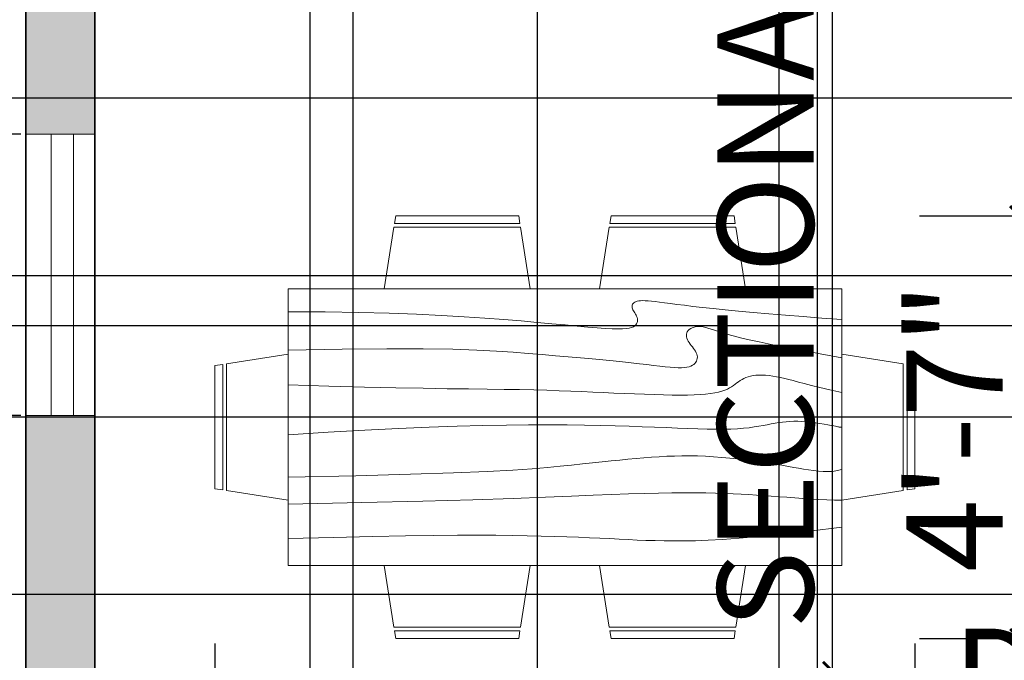
# Model space of a CAD drawing. Units: inches. Extents: x 1763 to 2368, y 1500 to 2097.
# Tile 6 of 24: x 1828 to 1956, y 1794 to 1877. Entities that reach past the tile are written whole.
import ezdxf

# ---------------------------------------------------------------- set-up
doc = ezdxf.new("R2010")
doc.units = ezdxf.units.IN
for name, color, linetype, lineweight in [('A-ANNO-DIMS', 2, 'Continuous', 18), ('A-FURN', 8, 'Continuous', 18), ('A-WALL', 7, 'Continuous', 35), ('A-WALL-PATT', 7, 'Continuous', 13), ('windows', 1, 'Continuous', 18)]:
    doc.layers.add(name, color=color, linetype=linetype, lineweight=lineweight)
doc.styles.get("Standard").update_dxf_attribs({"font": 'arial.ttf'})
doc.dimstyles.new('ISO-25', dxfattribs={"dimtxt": 12.5, "dimasz": 2.5, "dimexe": 1.25, "dimexo": 0.625, "dimtad": 1, "dimdec": 0, "dimlunit": 4, "dimtxsty": 'Standard', "dimblk": 'ARCHTICK', "dimcen": 2.5, "dimclrd": 3, "dimclrt": 4, "dimadec": 0, "dimazin": 0, "dimtfac": 1, "dimtdec": 0, "dimtmove": 0, "dimatfit": 3, "dimfxl": 1, "dimarcsym": 0})

# ---------------------------------------------------------------- blocks, each defined once
blk = doc.blocks.new('Dining Set - 36 x 72 in.')
for p, q in [((-22, 27.5), (-22.1562, 26.50042)), ((-22, 27.5), (-6, 27.5)), ((-5.8437, 26.49966), (-6, 27.5)), ((6, 27.5), (5.8438, 26.50042)), ((6, 27.5), (22, 27.5)), ((22.1563, 26.49966), (22, 27.5)), ((-22.2343, 26.00059), (-23.4847, 17.99762)), ((-22.2304, 26), (-5.7608, 26)), ((-5.8416, 26.5), (-22.1534, 26.5)), ((-4.5152, 17.99762), (-5.7655, 25.99926)), ((5.7657, 26.00059), (4.5153, 17.99762)), ((5.7696, 26), (22.2392, 26)), ((22.1584, 26.5), (5.8466, 26.5)), ((23.4848, 17.99762), (22.2345, 25.99926)), ((36, 18), (-36, 18)), ((-36, 18), (-36, -18)), ((36, -18), (36, 18)), ((-44.0006, 8.23428), (-35.9976, 9.48474)), ((44.0006, 8.23428), (35.9976, 9.48474)), ((-45.5, 8), (-44.5004, 8.15617)), ((-45.5, 8), (-45.5, -8)), ((-44.5, -8.15843), (-44.5, 8.15338)), ((-44, 8.23041), (-44, -8.23915)), ((44, 8.23041), (44, -8.23915)), ((44.5, -8.15843), (44.5, 8.15338)), ((45.5, 8), (44.5005, 8.15617)), ((45.5, 8), (45.5, -8)), ((-44.4997, -8.15631), (-45.5, -8)), ((-35.9976, -9.48476), (-43.9993, -8.2345)), ((35.9976, -9.48476), (43.9993, -8.2345)), ((44.4997, -8.15631), (45.5, -8)), ((-36, -18), (36, -18)), ((-22.2343, -26.0006), (-23.4847, -17.99762)), ((-4.5152, -17.99762), (-5.7655, -25.99928)), ((5.7657, -26.0006), (4.5153, -17.99762)), ((23.4848, -17.99762), (22.2345, -25.99928)), ((-22.2304, -26), (-5.7608, -26)), ((-22, -27.5), (-22.1562, -26.50044)), ((-5.8416, -26.5), (-22.1534, -26.5)), ((-5.8437, -26.49967), (-6, -27.5)), ((5.7696, -26), (22.2392, -26)), ((6, -27.5), (5.8438, -26.50044)), ((22.1584, -26.5), (5.8466, -26.5)), ((22.1563, -26.49967), (22, -27.5)), ((-22, -27.5), (-6, -27.5)), ((6, -27.5), (22, -27.5))]:
    blk.add_line(p, q)
for points in [[(-36, 15), (-31.1772, 14.97754), (-26.8079, 14.91406), (-22.8538, 14.81543), (-19.276, 14.6875), (-16.0362, 14.53613), (-13.0957, 14.36718), (-10.4159, 14.18652), (-7.9583, 14), (-5.6904, 13.81315), (-3.6035, 13.63021), (-1.6954, 13.45508), (0.0365, 13.29166), (1.5945, 13.14388), (2.9811, 13.01562), (4.1988, 12.9108), (5.25, 12.83333), (6.1393, 12.78613), (6.8802, 12.76823), (7.4883, 12.77767), (7.9792, 12.8125), (8.3685, 12.87077), (8.6719, 12.95052), (8.9049, 13.0498), (9.0833, 13.16666), (9.2205, 13.29899), (9.3216, 13.44401), (9.3895, 13.59879), (9.4271, 13.76041), (9.4373, 13.92594), (9.4232, 14.09245), (9.3875, 14.257), (9.3333, 14.41666), (9.2638, 14.56917), (9.1836, 14.71484), (9.0975, 14.85465), (9.0104, 14.98958), (8.9272, 15.1206), (8.8529, 15.2487), (8.7922, 15.37483), (8.75, 15.5), (8.7305, 15.62467), (8.7344, 15.74739), (8.7617, 15.86621), (8.8125, 15.97916), (8.8867, 16.08431), (8.9844, 16.17968), (9.1055, 16.26334), (9.25, 16.33333), (9.4189, 16.38802), (9.6172, 16.42708), (9.8506, 16.45052), (10.125, 16.45833), (10.4463, 16.45052), (10.8203, 16.42708), (11.2529, 16.38802), (11.75, 16.33333), (12.3184, 16.26318), (12.9694, 16.17838), (13.7151, 16.07991), (14.5677, 15.96875), (15.5395, 15.84586), (16.6426, 15.71224), (17.8893, 15.56884), (19.2917, 15.41666), (20.859, 15.25667), (22.5879, 15.08984), (24.4721, 14.91715), (26.5052, 14.73958), (28.6809, 14.5581), (30.9929, 14.3737), (33.4347, 14.18733), (36, 14)], [(-36, 10), (-28.9766, 10.14274), (-23.1725, 10.20442), (-18.4241, 10.19775), (-14.5677, 10.13541), (-11.4399, 10.03011), (-8.877, 9.89453), (-6.7154, 9.74137), (-4.7917, 9.58333), (-2.9698, 9.43082), (-1.2246, 9.28515), (0.4415, 9.14534), (2.026, 9.01041), (3.5266, 8.87939), (4.9408, 8.7513), (6.266, 8.62516), (7.5, 8.5), (8.6411, 8.37549), (9.6914, 8.2539), (10.6538, 8.13818), (11.5312, 8.03125), (12.3267, 7.93603), (13.043, 7.85547), (13.6831, 7.79248), (14.25, 7.75), (14.7471, 7.7303), (15.1797, 7.73307), (15.5537, 7.75732), (15.875, 7.80208), (16.1494, 7.86637), (16.3828, 7.94922), (16.5811, 8.04964), (16.75, 8.16666), (16.8944, 8.29915), (17.0143, 8.44531), (17.1089, 8.60319), (17.1771, 8.77083), (17.218, 8.94629), (17.2305, 9.1276), (17.2137, 9.31282), (17.1667, 9.5), (17.0895, 9.6875), (16.987, 9.875), (16.8649, 10.0625), (16.7292, 10.25), (16.5856, 10.4375), (16.4401, 10.625), (16.2985, 10.8125), (16.1667, 11), (16.05, 11.18733), (15.9518, 11.3737), (15.8752, 11.5581), (15.8229, 11.73958), (15.798, 11.91715), (15.8034, 12.08984), (15.842, 12.25667), (15.9167, 12.41666), (16.0295, 12.56836), (16.1784, 12.70833), (16.3605, 12.83268), (16.5729, 12.9375), (16.8127, 13.01888), (17.0768, 13.07291), (17.3625, 13.0957), (17.6667, 13.08333), (17.9894, 13.03312), (18.3418, 12.94726), (18.7382, 12.82918), (19.1927, 12.68229), (19.7195, 12.51001), (20.3327, 12.31575), (21.0465, 12.10294), (21.875, 11.875), (22.8357, 11.63354), (23.959, 11.37304), (25.2786, 11.08618), (26.8282, 10.76562), (28.6414, 10.40405), (30.752, 9.99414), (33.1936, 9.52856), (36, 9)], [(-36, 5.5), (-30.7157, 5.3348), (-26.069, 5.20963), (-21.9946, 5.11767), (-18.4271, 5.05208), (-15.3009, 5.00602), (-12.5508, 4.97265), (-10.1112, 4.94515), (-7.9167, 4.91666), (-5.909, 4.88167), (-4.0586, 4.83984), (-2.3429, 4.79215), (-0.7396, 4.73958), (0.7739, 4.6831), (2.22, 4.6237), (3.6213, 4.56233), (5, 4.5), (6.373, 4.43782), (7.7344, 4.3776), (9.0723, 4.32129), (10.375, 4.27083), (11.6309, 4.22819), (12.8281, 4.19531), (13.9551, 4.17415), (15, 4.16666), (15.954, 4.17448), (16.819, 4.19791), (17.6001, 4.23698), (18.3021, 4.29166), (18.9299, 4.36198), (19.4883, 4.44791), (19.9823, 4.54948), (20.4167, 4.66666), (20.7969, 4.79899), (21.1302, 4.94401), (21.4245, 5.09879), (21.6875, 5.26041), (21.9271, 5.42594), (22.1511, 5.59245), (22.3672, 5.757), (22.5834, 5.91666), (22.8065, 6.06868), (23.0404, 6.21093), (23.2879, 6.34147), (23.5521, 6.45833), (23.8358, 6.55957), (24.142, 6.64323), (24.4735, 6.70735), (24.8334, 6.75), (25.2235, 6.76969), (25.642, 6.76692), (26.0858, 6.74267), (26.5521, 6.69791), (27.0379, 6.63362), (27.5404, 6.55078), (28.0565, 6.45036), (28.5834, 6.33333), (29.1242, 6.19987), (29.7071, 6.04687), (30.3661, 5.87044), (31.1354, 5.66666), (32.0493, 5.43164), (33.142, 5.16146), (34.4475, 4.85221), (36, 4.5)], [(-36, -1), (-30.7915, -0.6591), (-26.0195, -0.38216), (-21.6519, -0.16284), (-17.6563, 0.00521), (-14.0005, 0.12833), (-10.6523, 0.21289), (-7.5796, 0.26522), (-4.75, 0.29166), (-2.134, 0.29793), (0.2878, 0.28711), (2.5317, 0.26163), (4.6146, 0.22396), (6.5529, 0.17651), (8.3633, 0.12174), (10.0623, 0.06209), (11.6667, 0), (13.1899, -0.06201), (14.6341, -0.1211), (15.9982, -0.17432), (17.2813, -0.21875), (18.4823, -0.25147), (19.6003, -0.26953), (20.6343, -0.27002), (21.5834, -0.25), (22.4481, -0.20768), (23.2357, -0.14584), (23.9549, -0.06836), (24.6146, 0.02083), (25.2235, 0.11784), (25.7904, 0.21875), (26.3241, 0.31966), (26.8334, 0.41666), (27.3265, 0.50618), (27.8099, 0.58593), (28.2894, 0.65397), (28.7709, 0.70833), (29.2601, 0.74707), (29.763, 0.76823), (30.2855, 0.76985), (30.8334, 0.75), (31.4088, 0.70784), (31.9994, 0.64713), (32.589, 0.57275), (33.1615, 0.48958), (33.7008, 0.4025), (34.1908, 0.3164), (34.6153, 0.23616), (34.9584, 0.16666), (35.2099, 0.11165), (35.3848, 0.07031), (35.504, 0.04069), (35.5886, 0.02083), (35.6594, 0.00879), (35.7377, 0.0026), (35.8442, 0.00032), (36, 0)], [(-36, -6.5), (-27.1843, -6.31267), (-20.084, -6.1263), (-14.469, -5.9419), (-10.1094, -5.76042), (-6.7752, -5.58285), (-4.2363, -5.41016), (-2.2629, -5.24333), (-0.625, -5.08334), (0.8708, -4.93099), (2.2715, -4.78646), (3.5872, -4.64974), (4.8281, -4.52084), (6.0046, -4.39974), (7.127, -4.28646), (8.2053, -4.18099), (9.25, -4.08334), (10.2705, -3.99382), (11.2734, -3.91407), (12.2647, -3.84603), (13.25, -3.79167), (14.2354, -3.75293), (15.2266, -3.73177), (16.2295, -3.73015), (17.25, -3.75), (18.2912, -3.79248), (19.3451, -3.85547), (20.4009, -3.93604), (21.4479, -4.03125), (22.4754, -4.13819), (23.4727, -4.25391), (24.4289, -4.37549), (25.3334, -4.5), (26.1785, -4.62492), (26.9694, -4.74935), (27.7145, -4.87281), (28.4219, -4.99479), (29.1, -5.11483), (29.7572, -5.23242), (30.4016, -5.34709), (31.0417, -5.45834), (31.6837, -5.56437), (32.3262, -5.65821), (32.9658, -5.73153), (33.599, -5.77604), (34.2224, -5.78345), (34.8327, -5.74545), (35.4264, -5.65373), (36, -5.5)], [(-36, -10), (-26.4022, -9.81299), (-18.4675, -9.62891), (-11.9839, -9.45069), (-6.7396, -9.28125), (-2.5226, -9.12354), (0.8789, -8.98047), (3.6769, -8.85498), (6.0833, -8.75), (8.2767, -8.66765), (10.3021, -8.60677), (12.1712, -8.56543), (13.8958, -8.54167), (15.4876, -8.53353), (16.9583, -8.53907), (18.3197, -8.55632), (19.5834, -8.58334), (20.7616, -8.61841), (21.8685, -8.66081), (22.9188, -8.71004), (23.9271, -8.76563), (24.9081, -8.82707), (25.8763, -8.89388), (26.8465, -8.96558), (27.8334, -9.04167), (28.8474, -9.12118), (29.8828, -9.20117), (30.93, -9.27824), (31.9792, -9.34896), (33.0205, -9.40991), (34.0443, -9.45768), (35.0407, -9.48885), (36, -9.5)], [(-36, -14.5), (-30.0881, -14.33513), (-25.0332, -14.21224), (-20.7312, -14.12647), (-17.0781, -14.07292), (-13.97, -14.04671), (-11.3027, -14.04297), (-8.9724, -14.05681), (-6.875, -14.08334), (-4.9224, -14.11833), (-3.0905, -14.16016), (-1.3709, -14.20785), (0.2448, -14.26042), (1.7647, -14.3169), (3.1973, -14.3763), (4.5507, -14.43767), (5.8333, -14.5), (7.0554, -14.5621), (8.235, -14.62175), (9.3922, -14.67652), (10.5469, -14.72396), (11.7192, -14.76164), (12.929, -14.78711), (14.1965, -14.79794), (15.5417, -14.79167), (16.9933, -14.76424), (18.6152, -14.70508), (20.4804, -14.60197), (22.6615, -14.44271), (25.2312, -14.21509), (28.2624, -13.9069), (31.8277, -13.50594), (36, -13)]]:
    blk.add_lwpolyline(points)
blk = doc.blocks.new('_ArchTick')
at = {"color": 0, "linetype": 'ByBlock', "const_width": 0.15}
blk.add_lwpolyline([(-0.5, -0.5), (0.5, 0.5)], dxfattribs=at)
blk = doc.blocks.new('*D25')
at = {"layer": 'A-ANNO-DIMS', "color": 3, "lineweight": -2, "transparency": 16777216}
for p, q in [((1934.01, 1792.31), (1934.01, 1981.61)), ((1934.01, 1660.94), (1934.01, 1792.31))]:
    blk.add_line(p, q, dxfattribs=at)
at = {"layer": 'A-ANNO-DIMS', "color": 0, "lineweight": -2, "transparency": 16777216}
for p, q in [((1953.09, 1792.31), (1932.76, 1792.31)), ((1953.09, 1660.94), (1932.76, 1660.94))]:
    blk.add_line(p, q, dxfattribs=at)
at = {"layer": 'Defpoints', "color": 0, "transparency": 16777216}
for p in [(1934.01, 1792.31), (1953.72, 1792.31), (1953.72, 1660.94)]:
    blk.add_point(p, dxfattribs=at)
at = {"layer": 'A-ANNO-DIMS', "color": 3, "lineweight": -2, "transparency": 16777216, "xscale": 2.5, "yscale": 2.5, "zscale": 2.5}
for p, rotation in [((1934.01, 1792.31), 90), ((1934.01, 1660.94), 270)]:
    blk.add_blockref('_ArchTick', p, dxfattribs=dict(at, rotation=rotation))
at = {"layer": 'A-ANNO-DIMS', "color": 4, "transparency": 16777216, "insert": (1926.92, 1888.21), "char_height": 12.5, "attachment_point": 5, "rotation": 90}
blk.add_mtext('SECTIONAL 10\'-11 1/2"', dxfattribs=at)
blk = doc.blocks.new('*D27')
at = {"layer": 'A-ANNO-DIMS', "color": 0, "lineweight": -2, "transparency": 16777216}
for p, q in [((1853.71, 1795.96), (1853.71, 1781.68)), ((1944.71, 1795.96), (1944.71, 1781.68))]:
    blk.add_line(p, q, dxfattribs=at)
at = {"layer": 'A-ANNO-DIMS', "color": 3, "lineweight": -2, "transparency": 16777216}
for p, q in [((1853.71, 1782.93), (1944.71, 1782.93)), ((1944.71, 1782.93), (2085.85, 1782.93))]:
    blk.add_line(p, q, dxfattribs=at)
at = {"layer": 'Defpoints', "color": 0, "transparency": 16777216}
for p in [(1853.71, 1796.58), (1944.71, 1796.58), (1944.71, 1782.93)]:
    blk.add_point(p, dxfattribs=at)
at = {"layer": 'A-ANNO-DIMS', "color": 3, "lineweight": -2, "transparency": 16777216, "xscale": 2.5, "yscale": 2.5, "zscale": 2.5, "rotation": 180}
blk.add_blockref('_ArchTick', (1853.71, 1782.93), dxfattribs=at)
at = {"layer": 'A-ANNO-DIMS', "color": 3, "lineweight": -2, "transparency": 16777216, "xscale": 2.5, "yscale": 2.5, "zscale": 2.5}
blk.add_blockref('_ArchTick', (1944.71, 1782.93), dxfattribs=at)
at = {"layer": 'A-ANNO-DIMS', "color": 4, "transparency": 16777216, "insert": (2016.53, 1790.02), "char_height": 12.5, "attachment_point": 5}
blk.add_mtext('DINING SET 7\'-7"', dxfattribs=at)
blk = doc.blocks.new('*D28')
at = {"layer": 'A-ANNO-DIMS', "color": 0, "lineweight": -2, "transparency": 16777216}
for p, q in [((1945.34, 1851.58), (1959.61, 1851.58)), ((1945.34, 1796.58), (1959.61, 1796.58))]:
    blk.add_line(p, q, dxfattribs=at)
at = {"layer": 'A-ANNO-DIMS', "color": 3, "lineweight": -2, "transparency": 16777216}
blk.add_line((1958.36, 1796.58), (1958.36, 1851.58), dxfattribs=at)
at = {"layer": 'Defpoints', "color": 0, "transparency": 16777216}
for p in [(1944.71, 1851.58), (1958.36, 1851.58), (1944.71, 1796.58)]:
    blk.add_point(p, dxfattribs=at)
at = {"layer": 'A-ANNO-DIMS', "color": 3, "lineweight": -2, "transparency": 16777216, "xscale": 2.5, "yscale": 2.5, "zscale": 2.5}
for p, rotation in [((1958.36, 1851.58), 90), ((1958.36, 1796.58), 270)]:
    blk.add_blockref('_ArchTick', p, dxfattribs=dict(at, rotation=rotation))
at = {"layer": 'A-ANNO-DIMS', "color": 4, "transparency": 16777216, "insert": (1951.49, 1824.08), "char_height": 12.5, "attachment_point": 5, "rotation": 90}
blk.add_mtext('4\'-7"', dxfattribs=at)
blk = doc.blocks.new('*D47')
at = {"layer": 'A-ANNO-DIMS', "color": 0, "lineweight": -2, "transparency": 16777216}
for p, q in [((1828.47, 1825.59), (1787.6, 1825.59)), ((1828.47, 1738.64), (1787.6, 1738.64))]:
    blk.add_line(p, q, dxfattribs=at)
at = {"layer": 'A-ANNO-DIMS', "color": 3, "lineweight": -2, "transparency": 16777216}
blk.add_line((1788.85, 1738.64), (1788.85, 1825.59), dxfattribs=at)
at = {"layer": 'Defpoints', "color": 0, "transparency": 16777216}
for p in [(1788.85, 1825.59), (1829.09, 1825.59), (1829.09, 1738.64)]:
    blk.add_point(p, dxfattribs=at)
at = {"layer": 'A-ANNO-DIMS', "color": 3, "lineweight": -2, "transparency": 16777216, "xscale": 2.5, "yscale": 2.5, "zscale": 2.5}
for p, rotation in [((1788.85, 1825.59), 90), ((1788.85, 1738.64), 270)]:
    blk.add_blockref('_ArchTick', p, dxfattribs=dict(at, rotation=rotation))
at = {"layer": 'A-ANNO-DIMS', "color": 4, "transparency": 16777216, "insert": (1781.84, 1782.12), "char_height": 12.5, "attachment_point": 5, "rotation": 90}
blk.add_mtext('7\'-3"', dxfattribs=at)
blk = doc.blocks.new('*D48')
at = {"layer": 'A-ANNO-DIMS', "color": 3, "lineweight": -2, "transparency": 16777216}
for p, q in [((1788.85, 1862.2), (1788.85, 1928.3)), ((1788.85, 1825.59), (1788.85, 1862.2))]:
    blk.add_line(p, q, dxfattribs=at)
at = {"layer": 'A-ANNO-DIMS', "color": 0, "lineweight": -2, "transparency": 16777216}
for p, q in [((1828.47, 1862.2), (1787.6, 1862.2)), ((1828.47, 1825.59), (1787.6, 1825.59))]:
    blk.add_line(p, q, dxfattribs=at)
at = {"layer": 'Defpoints', "color": 0, "transparency": 16777216}
for p in [(1788.85, 1862.2), (1829.09, 1862.2), (1829.09, 1825.59)]:
    blk.add_point(p, dxfattribs=at)
at = {"layer": 'A-ANNO-DIMS', "color": 3, "lineweight": -2, "transparency": 16777216, "xscale": 2.5, "yscale": 2.5, "zscale": 2.5}
for p, rotation in [((1788.85, 1862.2), 90), ((1788.85, 1825.59), 270)]:
    blk.add_blockref('_ArchTick', p, dxfattribs=dict(at, rotation=rotation))
at = {"layer": 'A-ANNO-DIMS', "color": 4, "transparency": 16777216, "insert": (1781.76, 1896.5), "char_height": 12.5, "attachment_point": 5, "rotation": 90}
blk.add_mtext('3\'-0 1/2"', dxfattribs=at)
blk = doc.blocks.new('*D49')
at = {"layer": 'A-ANNO-DIMS', "color": 0, "lineweight": -2, "transparency": 16777216}
for p, q in [((1828.47, 1913.1), (1787.6, 1913.1)), ((1828.47, 1862.2), (1787.6, 1862.2))]:
    blk.add_line(p, q, dxfattribs=at)
at = {"layer": 'A-ANNO-DIMS', "color": 3, "lineweight": -2, "transparency": 16777216}
blk.add_line((1788.85, 1862.2), (1788.85, 1913.1), dxfattribs=at)
at = {"layer": 'Defpoints', "color": 0, "transparency": 16777216}
for p in [(1788.85, 1913.1), (1829.09, 1913.1), (1829.09, 1862.2)]:
    blk.add_point(p, dxfattribs=at)
at = {"layer": 'A-ANNO-DIMS', "color": 3, "lineweight": -2, "transparency": 16777216, "xscale": 2.5, "yscale": 2.5, "zscale": 2.5}
for p, rotation in [((1788.85, 1913.1), 90), ((1788.85, 1862.2), 270)]:
    blk.add_blockref('_ArchTick', p, dxfattribs=dict(at, rotation=rotation))
at = {"layer": 'A-ANNO-DIMS', "color": 4, "transparency": 16777216, "insert": (1781.84, 1887.65), "char_height": 12.5, "attachment_point": 5, "rotation": 90}
blk.add_mtext('4\'-3"', dxfattribs=at)
blk = doc.blocks.new('*D58')
at = {"layer": 'A-ANNO-DIMS', "color": 0, "lineweight": -2, "transparency": 16777216}
for p, q in [((1871.68, 1635.9), (1871.68, 2072.02)), ((1927.07, 1635.9), (1927.07, 2072.02))]:
    blk.add_line(p, q, dxfattribs=at)
at = {"layer": 'A-ANNO-DIMS', "color": 3, "lineweight": -2, "transparency": 16777216}
for p, q in [((1871.68, 2070.77), (1927.07, 2070.77)), ((1927.07, 2070.77), (1993.68, 2070.77))]:
    blk.add_line(p, q, dxfattribs=at)
at = {"layer": 'Defpoints', "color": 0, "transparency": 16777216}
for p in [(1927.07, 2070.77), (1871.68, 1635.27), (1927.07, 1635.27)]:
    blk.add_point(p, dxfattribs=at)
at = {"layer": 'A-ANNO-DIMS', "color": 3, "lineweight": -2, "transparency": 16777216, "xscale": 2.5, "yscale": 2.5, "zscale": 2.5, "rotation": 180}
blk.add_blockref('_ArchTick', (1871.68, 2070.77), dxfattribs=at)
at = {"layer": 'A-ANNO-DIMS', "color": 3, "lineweight": -2, "transparency": 16777216, "xscale": 2.5, "yscale": 2.5, "zscale": 2.5}
blk.add_blockref('_ArchTick', (1927.07, 2070.77), dxfattribs=at)
at = {"layer": 'A-ANNO-DIMS', "color": 4, "transparency": 16777216, "insert": (1961.63, 2077.86), "char_height": 12.5, "attachment_point": 5}
blk.add_mtext('4\'-7 1/2"', dxfattribs=at)
blk = doc.blocks.new('*D68')
at = {"layer": 'A-ANNO-DIMS', "color": 0, "lineweight": -2, "transparency": 16777216}
for p, q in [((1895.59, 1879.65), (1895.59, 1509.91)), ((1932.01, 1879.65), (1932.01, 1509.91))]:
    blk.add_line(p, q, dxfattribs=at)
at = {"layer": 'A-ANNO-DIMS', "color": 3, "lineweight": -2, "transparency": 16777216}
for p, q in [((1895.59, 1511.16), (1932.01, 1511.16)), ((1932.01, 1511.16), (1998.11, 1511.16))]:
    blk.add_line(p, q, dxfattribs=at)
at = {"layer": 'Defpoints', "color": 0, "transparency": 16777216}
for p in [(1895.59, 1880.27), (1932.01, 1880.27), (1932.01, 1511.16)]:
    blk.add_point(p, dxfattribs=at)
at = {"layer": 'A-ANNO-DIMS', "color": 3, "lineweight": -2, "transparency": 16777216, "xscale": 2.5, "yscale": 2.5, "zscale": 2.5, "rotation": 180}
blk.add_blockref('_ArchTick', (1895.59, 1511.16), dxfattribs=at)
at = {"layer": 'A-ANNO-DIMS', "color": 3, "lineweight": -2, "transparency": 16777216, "xscale": 2.5, "yscale": 2.5, "zscale": 2.5}
blk.add_blockref('_ArchTick', (1932.01, 1511.16), dxfattribs=at)
at = {"layer": 'A-ANNO-DIMS', "color": 4, "transparency": 16777216, "insert": (1966.31, 1518.25), "char_height": 12.5, "attachment_point": 5}
blk.add_mtext('3\'-0 1/2"', dxfattribs=at)
blk = doc.blocks.new('*D69')
at = {"layer": 'A-ANNO-DIMS', "color": 0, "lineweight": -2, "transparency": 16777216}
for p, q in [((1838.09, 1879.65), (1838.09, 1509.91)), ((1895.59, 1879.65), (1895.59, 1509.91))]:
    blk.add_line(p, q, dxfattribs=at)
at = {"layer": 'A-ANNO-DIMS', "color": 3, "lineweight": -2, "transparency": 16777216}
for p, q in [((1838.09, 1511.16), (1895.59, 1511.16)), ((1895.59, 1511.16), (1962.2, 1511.16))]:
    blk.add_line(p, q, dxfattribs=at)
at = {"layer": 'Defpoints', "color": 0, "transparency": 16777216}
for p in [(1838.09, 1880.27), (1895.59, 1880.27), (1895.59, 1511.16)]:
    blk.add_point(p, dxfattribs=at)
at = {"layer": 'A-ANNO-DIMS', "color": 3, "lineweight": -2, "transparency": 16777216, "xscale": 2.5, "yscale": 2.5, "zscale": 2.5, "rotation": 180}
blk.add_blockref('_ArchTick', (1838.09, 1511.16), dxfattribs=at)
at = {"layer": 'A-ANNO-DIMS', "color": 3, "lineweight": -2, "transparency": 16777216, "xscale": 2.5, "yscale": 2.5, "zscale": 2.5}
blk.add_blockref('_ArchTick', (1895.59, 1511.16), dxfattribs=at)
at = {"layer": 'A-ANNO-DIMS', "color": 4, "transparency": 16777216, "insert": (1930.15, 1518.24), "char_height": 12.5, "attachment_point": 5}
blk.add_mtext('4\'-9 1/2"', dxfattribs=at)
blk = doc.blocks.new('*D79')
at = {"layer": 'A-ANNO-DIMS', "color": 3, "lineweight": -2, "transparency": 16777216}
for p, q in [((1788.85, 1825.4), (1788.85, 1870.91)), ((1788.85, 1802.3), (1788.85, 1825.4))]:
    blk.add_line(p, q, dxfattribs=at)
at = {"layer": 'A-ANNO-DIMS', "color": 0, "lineweight": -2, "transparency": 16777216}
for p, q in [((2054.47, 1825.4), (1787.6, 1825.4)), ((2054.47, 1802.3), (1787.6, 1802.3))]:
    blk.add_line(p, q, dxfattribs=at)
at = {"layer": 'Defpoints', "color": 0, "transparency": 16777216}
for p in [(1788.85, 1825.4), (2055.09, 1825.4), (2055.09, 1802.3)]:
    blk.add_point(p, dxfattribs=at)
at = {"layer": 'A-ANNO-DIMS', "color": 3, "lineweight": -2, "transparency": 16777216, "xscale": 2.5, "yscale": 2.5, "zscale": 2.5}
for p, rotation in [((1788.85, 1825.4), 90), ((1788.85, 1802.3), 270)]:
    blk.add_blockref('_ArchTick', p, dxfattribs=dict(at, rotation=rotation))
at = {"layer": 'A-ANNO-DIMS', "color": 4, "transparency": 16777216, "insert": (1781.95, 1849.4), "char_height": 12.5, "attachment_point": 5, "rotation": 90}
blk.add_mtext('1\'-11"', dxfattribs=at)
blk = doc.blocks.new('*D80')
at = {"layer": 'A-ANNO-DIMS', "color": 3, "lineweight": -2, "transparency": 16777216}
for p, q in [((1788.85, 1837.27), (1788.85, 1873.07)), ((1788.85, 1825.4), (1788.85, 1837.27))]:
    blk.add_line(p, q, dxfattribs=at)
at = {"layer": 'A-ANNO-DIMS', "color": 0, "lineweight": -2, "transparency": 16777216}
for p, q in [((2054.47, 1837.27), (1787.6, 1837.27)), ((2054.47, 1825.4), (1787.6, 1825.4))]:
    blk.add_line(p, q, dxfattribs=at)
at = {"layer": 'Defpoints', "color": 0, "transparency": 16777216}
for p in [(1788.85, 1837.27), (2055.09, 1837.27), (2055.09, 1825.4)]:
    blk.add_point(p, dxfattribs=at)
at = {"layer": 'A-ANNO-DIMS', "color": 3, "lineweight": -2, "transparency": 16777216, "xscale": 2.5, "yscale": 2.5, "zscale": 2.5}
for p, rotation in [((1788.85, 1837.27), 90), ((1788.85, 1825.4), 270)]:
    blk.add_blockref('_ArchTick', p, dxfattribs=dict(at, rotation=rotation))
at = {"layer": 'A-ANNO-DIMS', "color": 4, "transparency": 16777216, "insert": (1781.85, 1856.42), "char_height": 12.5, "attachment_point": 5, "rotation": 90}
blk.add_mtext('1\'-0"', dxfattribs=at)
blk = doc.blocks.new('*D81')
at = {"layer": 'A-ANNO-DIMS', "color": 3, "lineweight": -2, "transparency": 16777216}
for p, q in [((1788.85, 1866.87), (1788.85, 1912.38)), ((1788.85, 1843.77), (1788.85, 1866.87))]:
    blk.add_line(p, q, dxfattribs=at)
at = {"layer": 'A-ANNO-DIMS', "color": 0, "lineweight": -2, "transparency": 16777216}
for p, q in [((2077.47, 1866.87), (1787.6, 1866.87)), ((2077.47, 1843.77), (1787.6, 1843.77))]:
    blk.add_line(p, q, dxfattribs=at)
at = {"layer": 'Defpoints', "color": 0, "transparency": 16777216}
for p in [(1788.85, 1866.87), (2078.09, 1866.87), (2078.09, 1843.77)]:
    blk.add_point(p, dxfattribs=at)
at = {"layer": 'A-ANNO-DIMS', "color": 3, "lineweight": -2, "transparency": 16777216, "xscale": 2.5, "yscale": 2.5, "zscale": 2.5}
for p, rotation in [((1788.85, 1866.87), 90), ((1788.85, 1843.77), 270)]:
    blk.add_blockref('_ArchTick', p, dxfattribs=dict(at, rotation=rotation))
at = {"layer": 'A-ANNO-DIMS', "color": 4, "transparency": 16777216, "insert": (1781.95, 1890.87), "char_height": 12.5, "attachment_point": 5, "rotation": 90}
blk.add_mtext('1\'-11"', dxfattribs=at)
blk = doc.blocks.new('*D82')
at = {"layer": 'A-ANNO-DIMS', "color": 3, "lineweight": -2, "transparency": 16777216}
for p, q in [((1788.85, 1843.77), (1788.85, 1909.87)), ((1788.85, 1837.27), (1788.85, 1843.77))]:
    blk.add_line(p, q, dxfattribs=at)
at = {"layer": 'A-ANNO-DIMS', "color": 0, "lineweight": -2, "transparency": 16777216}
for p, q in [((2077.47, 1843.77), (1787.6, 1843.77)), ((2077.47, 1837.27), (1787.6, 1837.27))]:
    blk.add_line(p, q, dxfattribs=at)
at = {"layer": 'Defpoints', "color": 0, "transparency": 16777216}
for p in [(1788.85, 1843.77), (2078.09, 1843.77), (2078.09, 1837.27)]:
    blk.add_point(p, dxfattribs=at)
at = {"layer": 'A-ANNO-DIMS', "color": 3, "lineweight": -2, "transparency": 16777216, "xscale": 2.5, "yscale": 2.5, "zscale": 2.5}
for p, rotation in [((1788.85, 1843.77), 90), ((1788.85, 1837.27), 270)]:
    blk.add_blockref('_ArchTick', p, dxfattribs=dict(at, rotation=rotation))
at = {"layer": 'A-ANNO-DIMS', "color": 4, "transparency": 16777216, "insert": (1781.77, 1878.07), "char_height": 12.5, "attachment_point": 5, "rotation": 90}
blk.add_mtext('0\'-6 1/2"', dxfattribs=at)
blk = doc.blocks.new('*D90')
at = {"layer": 'A-ANNO-DIMS', "color": 0, "lineweight": -2, "transparency": 16777216}
for p, q in [((1838.09, 1980.65), (1838.09, 1509.91)), ((1866.04, 1955.7), (1866.04, 1509.91))]:
    blk.add_line(p, q, dxfattribs=at)
at = {"layer": 'A-ANNO-DIMS', "color": 3, "lineweight": -2, "transparency": 16777216}
for p, q in [((1838.09, 1511.16), (1866.04, 1511.16)), ((1866.04, 1511.16), (1903.23, 1511.16))]:
    blk.add_line(p, q, dxfattribs=at)
at = {"layer": 'Defpoints', "color": 0, "transparency": 16777216}
for p in [(1838.09, 1981.27), (1866.04, 1956.32), (1866.04, 1511.16)]:
    blk.add_point(p, dxfattribs=at)
at = {"layer": 'A-ANNO-DIMS', "color": 3, "lineweight": -2, "transparency": 16777216, "xscale": 2.5, "yscale": 2.5, "zscale": 2.5, "rotation": 180}
blk.add_blockref('_ArchTick', (1838.09, 1511.16), dxfattribs=at)
at = {"layer": 'A-ANNO-DIMS', "color": 3, "lineweight": -2, "transparency": 16777216, "xscale": 2.5, "yscale": 2.5, "zscale": 2.5}
blk.add_blockref('_ArchTick', (1866.04, 1511.16), dxfattribs=at)
at = {"layer": 'A-ANNO-DIMS', "color": 4, "transparency": 16777216, "insert": (1885.88, 1518.06), "char_height": 12.5, "attachment_point": 5}
blk.add_mtext('2\'-4"', dxfattribs=at)

msp = doc.modelspace()

# ---------------------------------------------------------------- hatches: boundary and pattern name
at = {"layer": 'A-WALL-PATT'}
h = msp.add_hatch(color=256, dxfattribs=at)
h.dxf.hatch_style = 1
h.paths.add_polyline_path([(1838.09, 2034.27), (1838.09, 2043.27), (1829.09, 2043.27), (1829.09, 1953.39), (1838.09, 1953.39)])
h.paths.add_polyline_path([(1838.09, 1913.1), (1829.09, 1913.1), (1829.09, 1862.2), (1838.09, 1862.2)])
h.paths.add_polyline_path([(1838.09, 1825.59), (1829.09, 1825.59), (1829.09, 1738.64), (1838.09, 1738.64)])
h.paths.add_polyline_path([(1895.59, 1885.27), (1838.09, 1885.27), (1838.09, 1880.27), (1895.59, 1880.27)])
h.paths.add_polyline_path([(1857.39, 1784.27), (1838.09, 1784.27), (1838.09, 1779.27), (1857.39, 1779.27)])
h.paths.add_polyline_path([(1958.09, 1981.27), (1971.46, 1981.27), (1971.46, 1986.27), (1968.57, 1986.27), (1958.09, 1986.27), (1953.09, 1986.27), (1927.39, 1986.27), (1927.39, 1981.27), (1953.09, 1981.27), (1953.09, 1885.27), (1932.01, 1885.27), (1932.01, 1880.27), (1959.13, 1880.27), (1959.13, 1883.74), (1959.13, 1885.27), (1958.09, 1885.27)])
h.paths.add_polyline_path([(2018.09, 1981.27), (2031.02, 1981.27), (2031.02, 1986.27), (2018.09, 1986.27), (2013.09, 1986.27), (2001.23, 1986.27), (2001.23, 1981.27), (2013.09, 1981.27), (2013.09, 1885.27), (1982.18, 1885.27, -0.016629), (1982.23, 1883.74), (1982.23, 1880.27), (2049.69, 1880.27), (2049.69, 1883.74, -0.016629), (2049.74, 1885.27), (2018.09, 1885.27)])
h.paths.add_polyline_path([(2083.09, 1981.27), (2120.61, 1981.27), (2120.61, 1986.27), (2083.09, 1986.27), (2078.09, 1986.27), (2063.14, 1986.27), (2063.14, 1981.27), (2078.09, 1981.27), (2078.09, 1885.27), (2072.78, 1885.27), (2072.78, 1883.74), (2072.78, 1880.27), (2078.09, 1880.27), (2078.09, 1866.87), (2081.56, 1866.87, -0.016629), (2083.09, 1866.82)])
h.paths.add_polyline_path([(1871.68, 1635.27), (1838.09, 1635.27), (1838.09, 1626.27), (1871.68, 1626.27)], flags=17)
h.paths.add_polyline_path([(2100.58, 1688.27), (2060.09, 1688.27), (2060.09, 1679.27), (2100.58, 1679.27)], flags=17)
h.paths.add_polyline_path([(2180.09, 1688.27), (2148.74, 1688.27), (2148.74, 1679.27), (2180.09, 1679.27)], flags=17)
h.paths.add_polyline_path([(2189.09, 1746.22), (2180.09, 1746.22), (2180.09, 1743.42), (2180.12, 1743.42), (2180.12, 1726.72), (2180.09, 1572.27), (2034.91, 1572.27), (2034.91, 1565.6), (2034.91, 1563.27), (2189.09, 1563.27)])
h.paths.add_polyline_path([(2060.09, 1802.35, -0.016629), (2058.56, 1802.3), (2055.09, 1802.3), (2055.09, 1635.27), (2042.48, 1635.27), (2042.48, 1629.74), (2042.48, 1626.27), (2055.09, 1626.27), (2055.09, 1599.27), (2040.27, 1599.27), (2040.27, 1590.27), (2060.09, 1590.27)])
h.paths.add_polyline_path([(2019.39, 1629.74, -0.060569), (2020.06, 1635.27), (1995.09, 1635.27), (1990.09, 1635.27), (1927.07, 1635.27), (1927.07, 1626.27), (1990.09, 1626.27), (1990.09, 1590.27), (1995.09, 1590.27), (2005.2, 1590.27), (2005.2, 1599.27), (1995.09, 1599.27), (1995.09, 1626.27), (2019.39, 1626.27)])
edge = h.paths.add_edge_path()
edge.add_line((2180.09, 1837.27), (2167.2, 1837.27))
edge.add_spline(control_points=[(2167.2, 1837.27), (2167.19, 1837.27), (2167.18, 1837.27), (2167.18, 1837.27)], knot_values=[168.955493, 168.955493, 168.955493, 168.955493, 169.065871, 169.065871, 169.065871, 169.065871], degree=3, periodic=0)
edge.add_spline(control_points=[(2167.18, 1837.27), (2166.56, 1837.38), (2166.33, 1846.16), (2165.71, 1846.24)], knot_values=[159.864705, 159.864705, 159.864705, 159.864705, 168.955493, 168.955493, 168.955493, 168.955493], degree=3, periodic=0)
edge.add_line((2167.12, 1837.27), (2163.16, 1837.27))
edge.add_spline(control_points=[(2163.16, 1837.27), (2163.16, 1837.27), (2163.16, 1837.27), (2163.15, 1837.27)], knot_values=[150.537172, 150.537172, 150.537172, 150.537172, 150.553797, 150.553797, 150.553797, 150.553797], degree=3, periodic=0)
edge.add_spline(control_points=[(2163.15, 1837.27), (2162.29, 1837.29), (2161.59, 1846.23), (2160.88, 1846.24)], knot_values=[141.293426, 141.293426, 141.293426, 141.293426, 150.537172, 150.537172, 150.537172, 150.537172], degree=3, periodic=0)
edge.add_line((2163.08, 1837.27), (2158.7, 1837.27))
edge.add_spline(control_points=[(2158.7, 1837.27), (2158.7, 1837.27), (2158.7, 1837.27), (2158.7, 1837.27)], knot_values=[132.033544, 132.033544, 132.033544, 132.033544, 132.049151, 132.049151, 132.049151, 132.049151], degree=3, periodic=0)
edge.add_spline(control_points=[(2158.7, 1837.27), (2157.97, 1837.29), (2157.26, 1846.23), (2156.39, 1846.24)], knot_values=[122.786021, 122.786021, 122.786021, 122.786021, 132.033544, 132.033544, 132.033544, 132.033544], degree=3, periodic=0)
edge.add_line((2158.63, 1837.27), (2153.84, 1837.27))
edge.add_spline(control_points=[(2153.84, 1837.27), (2153.83, 1837.27), (2153.82, 1837.27), (2153.82, 1837.27)], knot_values=[113.451585, 113.451585, 113.451585, 113.451585, 113.562103, 113.562103, 113.562103, 113.562103], degree=3, periodic=0)
edge.add_spline(control_points=[(2153.82, 1837.27), (2153.17, 1837.38), (2152.88, 1846.19), (2152.4, 1846.24)], knot_values=[0, 0, 0, 0, 9.081854, 9.081854, 9.081854, 9.081854], degree=3, periodic=0)
edge.add_line((2153.76, 1837.27), (2150.39, 1837.27))
edge.add_spline(control_points=[(2150.39, 1837.27), (2150.38, 1837.27), (2150.37, 1837.27), (2150.36, 1837.27)], knot_values=[95.069382, 95.069382, 95.069382, 95.069382, 95.17519, 95.17519, 95.17519, 95.17519], degree=3, periodic=0)
edge.add_spline(control_points=[(2150.36, 1837.27), (2149.49, 1837.37), (2148.42, 1846.19), (2147.59, 1846.24)], knot_values=[85.824599, 85.824599, 85.824599, 85.824599, 95.069382, 95.069382, 95.069382, 95.069382], degree=3, periodic=0)
edge.add_line((2150.29, 1837.27), (2145.43, 1837.27))
edge.add_spline(control_points=[(2145.43, 1837.27), (2145.43, 1837.27), (2145.42, 1837.27), (2145.42, 1837.27)], knot_values=[76.505559, 76.505559, 76.505559, 76.505559, 76.547811, 76.547811, 76.547811, 76.547811], degree=3, periodic=0)
edge.add_spline(control_points=[(2145.42, 1837.27), (2144.68, 1837.31), (2143.8, 1846.19), (2142.95, 1846.24)], knot_values=[67.23945, 67.23945, 67.23945, 67.23945, 76.505559, 76.505559, 76.505559, 76.505559], degree=3, periodic=0)
edge.add_line((2145.35, 1837.27), (2134.57, 1837.27))
edge.add_spline(control_points=[(2134.57, 1837.27), (2134.57, 1837.27), (2134.56, 1837.27), (2134.56, 1837.27)], knot_values=[39.001463, 39.001463, 39.001463, 39.001463, 39.045107, 39.045107, 39.045107, 39.045107], degree=3, periodic=0)
edge.add_spline(control_points=[(2134.56, 1837.27), (2133.87, 1837.31), (2133.4, 1845.85), (2132.33, 1846.24)], knot_values=[29.79778, 29.79778, 29.79778, 29.79778, 39.001463, 39.001463, 39.001463, 39.001463], degree=3, periodic=0)
edge.add_line((2134.5, 1837.27), (2128.08, 1837.27))
edge.add_spline(control_points=[(2128.08, 1837.27), (2128.03, 1837.26), (2127.98, 1837.26), (2127.93, 1837.27)], knot_values=[19.482067, 19.482067, 19.482067, 19.482067, 19.869396, 19.869396, 19.869396, 19.869396], degree=3, periodic=0)
edge.add_spline(control_points=[(2125.01, 1846.24), (2126.16, 1844.66), (2126.82, 1837.57), (2127.93, 1837.27)], knot_values=[10.389805, 10.389805, 10.389805, 10.389805, 19.482067, 19.482067, 19.482067, 19.482067], degree=3, periodic=0)
edge.add_line((2127.93, 1837.27), (2083.09, 1837.27))
edge.add_line((2083.09, 1837.27), (2083.09, 1843.77))
edge.add_line((2083.09, 1843.77), (2081.56, 1843.77))
edge.add_line((2081.56, 1843.77), (2078.09, 1843.77))
edge.add_line((2078.09, 1843.77), (2078.09, 1837.27))
edge.add_line((2078.09, 1837.27), (2055.09, 1837.27))
edge.add_line((2055.09, 1837.27), (2055.09, 1825.4))
edge.add_line((2055.09, 1825.4), (2058.56, 1825.4))
edge.add_line((2058.56, 1825.4), (2060.09, 1825.4))
edge.add_line((2060.09, 1825.4), (2060.09, 1832.27))
edge.add_line((2060.09, 1832.27), (2122.44, 1832.27))
edge.add_spline(control_points=[(2122.44, 1832.27), (2122.73, 1832.58), (2123.01, 1832.62), (2123.28, 1832.27)], knot_values=[5.972033, 5.972033, 5.972033, 5.972033, 8.057258, 8.057258, 8.057258, 8.057258], degree=3, periodic=0)
edge.add_line((2123.28, 1832.27), (2137.95, 1832.27))
edge.add_spline(control_points=[(2137.95, 1832.27), (2137.96, 1832.27), (2137.97, 1832.27), (2137.98, 1832.27)], knot_values=[53.926862, 53.926862, 53.926862, 53.926862, 54.030075, 54.030075, 54.030075, 54.030075], degree=3, periodic=0)
edge.add_spline(control_points=[(2139.72, 1825.02), (2139.28, 1825.06), (2138.67, 1832.18), (2137.98, 1832.27)], knot_values=[54.030075, 54.030075, 54.030075, 54.030075, 61.445194, 61.445194, 61.445194, 61.445194], degree=3, periodic=0)
edge.add_line((2138.05, 1832.27), (2140.96, 1832.27))
edge.add_spline(control_points=[(2140.96, 1832.27), (2140.97, 1832.27), (2140.98, 1832.27), (2140.99, 1832.27)], knot_values=[68.854182, 68.854182, 68.854182, 68.854182, 68.971237, 68.971237, 68.971237, 68.971237], degree=3, periodic=0)
edge.add_spline(control_points=[(2143.19, 1825.02), (2142.44, 1825.07), (2141.56, 1832.16), (2140.99, 1832.27)], knot_values=[68.971237, 68.971237, 68.971237, 68.971237, 76.444911, 76.444911, 76.444911, 76.444911], degree=3, periodic=0)
edge.add_line((2141.04, 1832.27), (2145.43, 1832.27))
edge.add_spline(control_points=[(2145.43, 1832.27), (2145.44, 1832.27), (2145.45, 1832.27), (2145.46, 1832.27)], knot_values=[84.039047, 84.039047, 84.039047, 84.039047, 84.124041, 84.124041, 84.124041, 84.124041], degree=3, periodic=0)
edge.add_spline(control_points=[(2148.11, 1825.02), (2147.34, 1825.02), (2146.3, 1832.19), (2145.46, 1832.27)], knot_values=[84.124041, 84.124041, 84.124041, 84.124041, 91.773891, 91.773891, 91.773891, 91.773891], degree=3, periodic=0)
edge.add_line((2145.54, 1832.27), (2150.39, 1832.27))
edge.add_spline(control_points=[(2150.39, 1832.27), (2150.42, 1832.28), (2150.45, 1832.28), (2150.47, 1832.27)], knot_values=[99.381577, 99.381577, 99.381577, 99.381577, 99.573457, 99.573457, 99.573457, 99.573457], degree=3, periodic=0)
edge.add_spline(control_points=[(2153.97, 1825.02), (2153.09, 1825.28), (2151.53, 1832.1), (2150.47, 1832.27)], knot_values=[99.573457, 99.573457, 99.573457, 99.573457, 107.218357, 107.218357, 107.218357, 107.218357], degree=3, periodic=0)
edge.add_line((2150.57, 1832.27), (2155.6, 1832.27))
edge.add_spline(control_points=[(2155.6, 1832.27), (2155.6, 1832.27), (2155.61, 1832.27), (2155.62, 1832.27)], knot_values=[114.933058, 114.933058, 114.933058, 114.933058, 115.013624, 115.013624, 115.013624, 115.013624], degree=3, periodic=0)
edge.add_spline(control_points=[(2158.28, 1825.02), (2157.4, 1825.07), (2156.25, 1832.2), (2155.62, 1832.27)], knot_values=[115.013624, 115.013624, 115.013624, 115.013624, 122.616269, 122.616269, 122.616269, 122.616269], degree=3, periodic=0)
edge.add_line((2155.68, 1832.27), (2165.19, 1832.27))
edge.add_spline(control_points=[(2165.19, 1832.27), (2165.2, 1832.27), (2165.2, 1832.27), (2165.2, 1832.27)], knot_values=[145.488477, 145.488477, 145.488477, 145.488477, 145.516379, 145.516379, 145.516379, 145.516379], degree=3, periodic=0)
edge.add_spline(control_points=[(2167.45, 1825.02), (2166.96, 1825.02), (2166.06, 1832.25), (2165.2, 1832.27)], knot_values=[145.516379, 145.516379, 145.516379, 145.516379, 153.105469, 153.105469, 153.105469, 153.105469], degree=3, periodic=0)
edge.add_line((2165.29, 1832.27), (2168.93, 1832.27))
edge.add_spline(control_points=[(2168.93, 1832.27), (2168.98, 1832.29), (2169.04, 1832.29), (2169.1, 1832.27)], knot_values=[160.517439, 160.517439, 160.517439, 160.517439, 160.939723, 160.939723, 160.939723, 160.939723], degree=3, periodic=0)
edge.add_spline(control_points=[(2171.09, 1828.64), (2170.35, 1830.37), (2169.62, 1832.09), (2169.1, 1832.27)], knot_values=[160.939723, 160.939723, 160.939723, 160.939723, 164.738835, 164.738835, 164.738835, 164.738835], degree=3, periodic=0)
edge.add_line((2169.1, 1832.27), (2180.09, 1832.27))
edge.add_line((2180.09, 1832.27), (2180.09, 1837.27))
h.paths.add_polyline_path([(2189.09, 1885.52), (2180.09, 1885.52), (2180.09, 1813.32), (2180.12, 1813.32), (2180.12, 1796.62), (2180.12, 1795.26), (2189.09, 1795.26)])
h.paths.add_polyline_path([(2180.09, 1986.27), (2166.28, 1986.27), (2166.28, 1981.27), (2180.09, 1981.27)])
h.paths.add_polyline_path([(2189.09, 2043.27), (2180.09, 2043.27), (2180.09, 2034.27), (2180.09, 1934.11), (2189.09, 1934.11)])
h.paths.add_polyline_path([(1838.09, 1681.59), (1829.09, 1681.59), (1829.09, 1563.27), (2003.86, 1563.27), (2003.86, 1565.6), (2003.86, 1572.27), (1838.09, 1572.27)])

# ---------------------------------------------------------------- linework, layer by layer
at = {"layer": 'A-WALL'}
msp.add_line((1838.09, 1572.27), (1838.09, 2034.27), dxfattribs=at)
msp.add_lwpolyline([(2003.86, 1563.27), (1829.09, 1563.27), (1829.09, 2043.27), (2189.09, 2043.27), (2189.09, 1563.27), (2034.91, 1563.27)], dxfattribs=at)
at = {"layer": 'windows'}
for p, q in [((1838.09, 1862.2), (1829.09, 1862.2)), ((1829.09, 1862.2), (1829.09, 1825.59)), ((1832.41, 1825.59), (1832.41, 1862.2)), ((1835.31, 1825.59), (1835.31, 1862.2)), ((1838.09, 1825.59), (1838.09, 1862.2)), ((1829.09, 1825.59), (1838.09, 1825.59))]:
    msp.add_line(p, q, dxfattribs=at)

# ---------------------------------------------------------------- block references
at = {"layer": 'A-FURN'}
msp.add_blockref('Dining Set - 36 x 72 in.', (1899.21, 1824.08), dxfattribs=at)

# ---------------------------------------------------------------- dimensions: what is measured, and where the dimension line sits
at = {"layer": 'A-ANNO-DIMS'}
for base, p1, p2, picture, middle in [((1927.07, 2070.77), (1871.68, 1635.27), (1927.07, 1635.27), '*D58', (1961.63, 2077.86)), ((1866.0388, 1511.1561), (1838.0918, 1981.2727), (1866.0388, 1956.3234), '*D90', (1885.8845, 1518.0567)), ((1895.59, 1511.16), (1838.09, 1880.27), (1895.59, 1880.27), '*D69', (1930.15, 1518.24)), ((1932.01, 1511.16), (1895.59, 1880.27), (1932.01, 1880.27), '*D68', (1966.31, 1518.25))]:
    dim = msp.add_linear_dim(base=base, p1=p1, p2=p2, dimstyle='ISO-25', override={"dimdec": 1, "dimlfac": 1, "dimrnd": 0, "dimzin": 1, "dimdsep": 46, "dimlunit": 4, "dimfrac": 2}, dxfattribs=at)
    dim.commit()
    dim.dimension.update_dxf_attribs({"geometry": picture, "text_midpoint": middle})
dim = msp.add_linear_dim(base=(1934.01, 1792.31), p1=(1953.72, 1660.94), p2=(1953.72, 1792.31), angle=90, text='SECTIONAL <>', dimstyle='ISO-25', override={"dimdec": 1, "dimlfac": 1, "dimrnd": 0, "dimzin": 1, "dimdsep": 46, "dimlunit": 4, "dimfrac": 2}, dxfattribs=at)
dim.commit()
dim.dimension.update_dxf_attribs({"geometry": '*D25', "text_midpoint": (1926.92, 1888.21)})
for base, p1, p2, picture, middle in [((1788.85, 1862.2), (1829.09, 1825.59), (1829.09, 1862.2), '*D48', (1781.76, 1896.5)), ((1788.85, 1913.1), (1829.09, 1862.2), (1829.09, 1913.1), '*D49', (1781.84, 1887.65)), ((1788.85, 1866.87), (2078.09, 1843.77), (2078.09, 1866.87), '*D81', (1781.95, 1890.87)), ((1788.85, 1843.77), (2078.09, 1837.27), (2078.09, 1843.77), '*D82', (1781.77, 1878.07)), ((1788.85, 1837.27), (2055.09, 1825.4), (2055.09, 1837.27), '*D80', (1781.85, 1856.42)), ((1788.85, 1825.4), (2055.09, 1802.3), (2055.09, 1825.4), '*D79', (1781.95, 1849.4)), ((1958.36, 1851.58), (1944.71, 1796.58), (1944.71, 1851.58), '*D28', (1951.49, 1824.08)), ((1788.8549, 1825.5896), (1829.0918, 1738.6434), (1829.0918, 1825.5896), '*D47', (1781.8435, 1782.1165))]:
    dim = msp.add_linear_dim(base=base, p1=p1, p2=p2, angle=90, dimstyle='ISO-25', override={"dimdec": 1, "dimlfac": 1, "dimrnd": 0, "dimzin": 1, "dimdsep": 46, "dimlunit": 4, "dimfrac": 2}, dxfattribs=at)
    dim.commit()
    dim.dimension.update_dxf_attribs({"geometry": picture, "text_midpoint": middle})
dim = msp.add_linear_dim(base=(1944.71, 1782.93), p1=(1853.71, 1796.58), p2=(1944.71, 1796.58), text='DINING SET <>', dimstyle='ISO-25', override={"dimdec": 1, "dimlfac": 1, "dimrnd": 0, "dimzin": 1, "dimdsep": 46, "dimlunit": 4, "dimfrac": 2}, dxfattribs=at)
dim.commit()
dim.dimension.update_dxf_attribs({"geometry": '*D27', "text_midpoint": (2016.53, 1790.02)})

doc.saveas('drawing.dxf')
